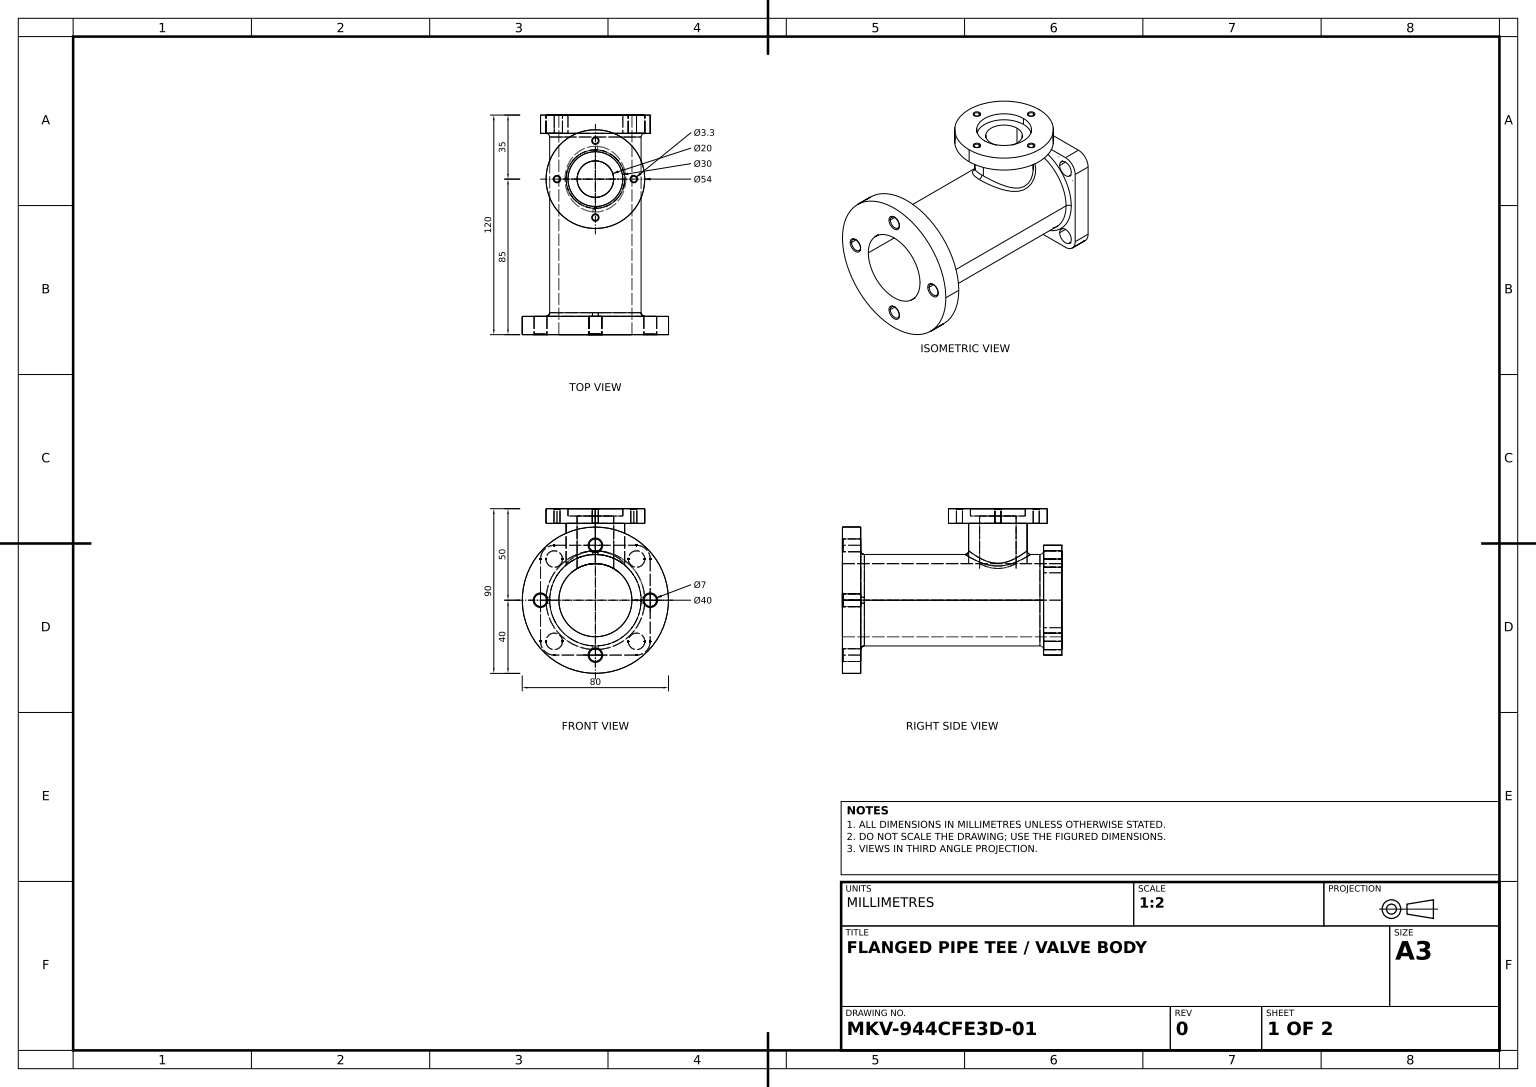
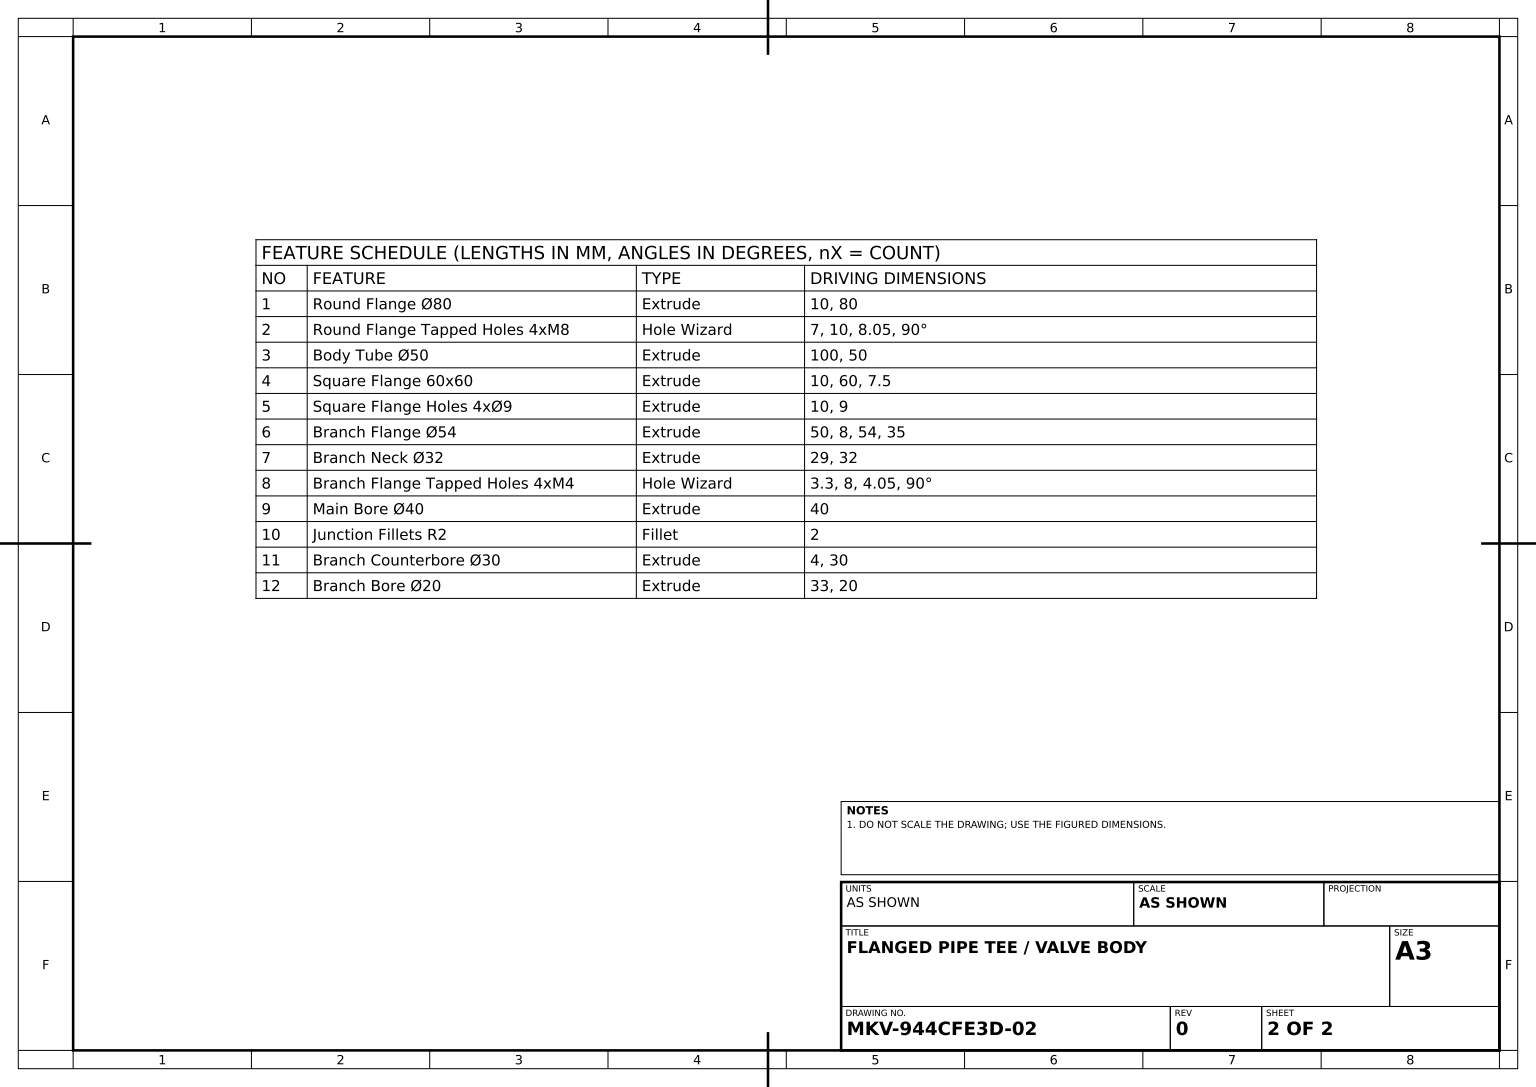
from build123d import *

# Parameters (mm, degrees)
ROUND_FLANGE_SKETCH_R                       = 40
ROUND_FLANGE_80_DEPTH                       = 10
ROUND_FLANGE_TAPPED_HOLES_4XM8_D            = 7
ROUND_FLANGE_TAPPED_HOLES_4XM8_CSINK_D      = 8.05
ROUND_FLANGE_TAPPED_HOLES_4XM8_CSINK_ANGLE  = 90
BODY_TUBE_SKETCH_R                          = 25
BODY_TUBE_50_DEPTH                          = 100
SQUARE_FLANGE_60X60_DEPTH                   = 10
SQUARE_FLANGE_HOLES_SKETCH_R                = 4.5
SQUARE_FLANGE_HOLES_4X_9_DEPTH              = 10
BRANCH_FLANGE_SKETCH_R                      = 27
BRANCH_FLANGE_54_DEPTH                      = 8
BRANCH_NECK_SKETCH_R                        = 16
BRANCH_NECK_32_DEPTH                        = 29
BRANCH_FLANGE_TAPPED_HOLES_4XM4_D           = 3.3
BRANCH_FLANGE_TAPPED_HOLES_4XM4_DEPTH       = 8
BRANCH_FLANGE_TAPPED_HOLES_4XM4_CSINK_D     = 4.05
BRANCH_FLANGE_TAPPED_HOLES_4XM4_CSINK_ANGLE = 90
MAIN_BORE_SKETCH_R                          = 20
MAIN_BORE_40_DEPTH                          = 137.014705087
JUNCTION_FILLETS_R2_R                       = 2
BRANCH_COUNTERBORE_SKETCH_R                 = 15
BRANCH_COUNTERBORE_30_DEPTH                 = 4
BRANCH_BORE_SKETCH_R                        = 10
BRANCH_BORE_20_DEPTH                        = 33


with BuildPart() as part:
    # Round Flange Sketch → Round Flange Ø80 (new body)
    with BuildSketch(Plane.XY):
        Circle(ROUND_FLANGE_SKETCH_R)
    extrude(amount=ROUND_FLANGE_80_DEPTH)

    # Round Flange Tapped Holes 4xM8 (through all)
    with Locations(Plane(origin=(-30, 0, 10), x_dir=(1, 0, 0), z_dir=(0, 0, 1))):
        with Locations((0, 0), (60, 0), (30, 30), (30, -30)):
            CounterSinkHole(ROUND_FLANGE_TAPPED_HOLES_4XM8_D / 2, ROUND_FLANGE_TAPPED_HOLES_4XM8_CSINK_D / 2, counter_sink_angle=ROUND_FLANGE_TAPPED_HOLES_4XM8_CSINK_ANGLE)

    # Body Tube Sketch → Body Tube Ø50 (add)
    with BuildSketch(Plane(origin=(0, 0, 0), x_dir=(-1, 0, 0), z_dir=(0, 0, -1))):
        Circle(BODY_TUBE_SKETCH_R)
    extrude(amount=BODY_TUBE_50_DEPTH)

    # Square Flange Sketch → Square Flange 60x60 (add)
    with BuildSketch(Plane(origin=(0, 0, -100), x_dir=(-1, 0, 0), z_dir=(0, 0, -1))):
        with BuildLine():
            Line((-22.5, -30), (22.5, -30))
            ThreePointArc((22.5, -30), (27.803300859, -27.803300859), (30, -22.5))
            Line((30, -22.5), (30, 22.5))
            ThreePointArc((30, 22.5), (27.803300859, 27.803300859), (22.5, 30))
            Line((22.5, 30), (-22.5, 30))
            ThreePointArc((-22.5, 30), (-27.803300859, 27.803300859), (-30, 22.5))
            Line((-30, 22.5), (-30, -22.5))
            ThreePointArc((-30, -22.5), (-27.803300859, -27.803300859), (-22.5, -30))
        make_face()
    extrude(amount=SQUARE_FLANGE_60X60_DEPTH)

    # Square Flange Holes Sketch → Square Flange Holes 4xØ9 (cut)
    with BuildSketch(Plane(origin=(0, 0, -110), x_dir=(-1, 0, 0), z_dir=(0, 0, -1))):
        with Locations((22.5, 22.5)):
            Circle(SQUARE_FLANGE_HOLES_SKETCH_R)
        with Locations((22.5, -22.5)):
            Circle(SQUARE_FLANGE_HOLES_SKETCH_R)
        with Locations((-22.5, -22.5)):
            Circle(SQUARE_FLANGE_HOLES_SKETCH_R)
        with Locations((-22.5, 22.5)):
            Circle(SQUARE_FLANGE_HOLES_SKETCH_R)
    extrude(amount=-SQUARE_FLANGE_HOLES_4X_9_DEPTH, mode=Mode.SUBTRACT)



with BuildPart() as body_2:
    # Branch Flange Sketch → Branch Flange Ø54 (new body)
    with BuildSketch(Plane(origin=(0, 50, 0), x_dir=(1, 0, 0), z_dir=(0, 1, 0))):
        with Locations(Location((0, 75, 0), (0, 0, 270))):
            Circle(BRANCH_FLANGE_SKETCH_R)
    extrude(amount=-BRANCH_FLANGE_54_DEPTH)


with BuildPart() as part_1:
    add(part.part)

    add(body_2.part)  # Branch Neck Ø32 merges body 2
    # Branch Neck Sketch → Branch Neck Ø32 (add)
    with BuildSketch(Plane.XZ.offset(-42)):
        with Locations(Location((0, -75, 0), (0, 0, 90))):
            Circle(BRANCH_NECK_SKETCH_R)
    extrude(amount=BRANCH_NECK_32_DEPTH)

    # Branch Flange Tapped Holes 4xM4
    with Locations(Plane(origin=(0, 50, -96), x_dir=(0, 0, 1), z_dir=(0, 1, 0))):
        with Locations((0, 0), (21, -21), (42, 0), (21, 21)):
            CounterSinkHole(BRANCH_FLANGE_TAPPED_HOLES_4XM4_D / 2, BRANCH_FLANGE_TAPPED_HOLES_4XM4_CSINK_D / 2, depth=BRANCH_FLANGE_TAPPED_HOLES_4XM4_DEPTH, counter_sink_angle=BRANCH_FLANGE_TAPPED_HOLES_4XM4_CSINK_ANGLE)

    # Main Bore Sketch → Main Bore Ø40 (cut, through all)
    with BuildSketch(Plane.XY.offset(10)):
        Circle(MAIN_BORE_SKETCH_R)
    extrude(amount=-MAIN_BORE_40_DEPTH, mode=Mode.SUBTRACT)

    # Junction Fillets R2
    junction_fillets_r2_edges = [part_1.edges().sort_by_distance(p)[0] for p in [
        (25, 0, 0),
        (25, 0, -100),
        (0, 25, -91),
    ]]
    fillet(junction_fillets_r2_edges, radius=JUNCTION_FILLETS_R2_R)

    # Branch Counterbore Sketch → Branch Counterbore Ø30 (cut)
    with BuildSketch(Plane(origin=(0, 50, 0), x_dir=(1, 0, 0), z_dir=(0, 1, 0))):
        with Locations(Location((0, 75, 0), (0, 0, 270))):
            Circle(BRANCH_COUNTERBORE_SKETCH_R)
    extrude(amount=-BRANCH_COUNTERBORE_30_DEPTH, mode=Mode.SUBTRACT)

    # Branch Bore Sketch → Branch Bore Ø20 (cut)
    with BuildSketch(Plane(origin=(0, 46, 0), x_dir=(1, 0, 0), z_dir=(0, 1, 0))):
        with Locations(Location((0, 75, 0), (0, 0, 270))):
            Circle(BRANCH_BORE_SKETCH_R)
    extrude(amount=-BRANCH_BORE_20_DEPTH, mode=Mode.SUBTRACT)


solid = part_1.part
